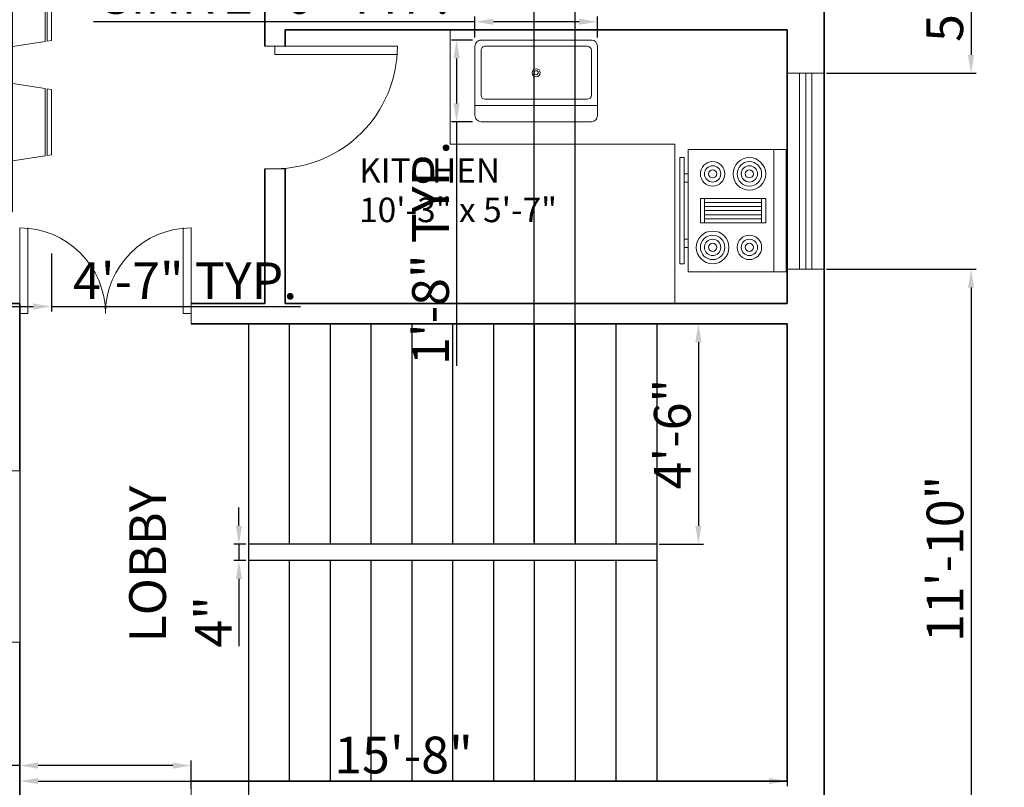
# Model space of a CAD drawing. Units: inches. Extents: x 3087 to 8148, y 1377 to 3709.
# Tile 5 of 6: x 3443 to 3684, y 1689 to 1877. Entities that reach past the tile are written whole.
import ezdxf

# ---------------------------------------------------------------- set-up
doc = ezdxf.new("R2010")
doc.units = ezdxf.units.IN
for name, color, linetype, lineweight, true_color in [('A-ANNO-DIMS', 244, 'Continuous', 18, 0x991b1e), ('A-AREA-IDEN', 244, 'Continuous', 18, 0x991b1e), ('A-DOOR', 146, 'Continuous', 18, 0x105689), ('A-FLOR-STRS', 146, 'Continuous', 25, 0x105689), ('A-GLAZ', 146, 'Continuous', 18, 0x105689), ('A-WALL', 241, 'Continuous', 35, 0xf7abae)]:
    doc.layers.add(name, color=color, linetype=linetype, lineweight=lineweight, true_color=true_color)
for name, color, linetype, lineweight in [('A-EQPM', 8, 'Continuous', 18), ('A-FLOR-CASE', 9, 'Continuous', 18), ('A-FLOR-FIXT', 9, 'Continuous', 18), ('A-FURN', 8, 'Continuous', 18)]:
    doc.layers.add(name, color=color, linetype=linetype, lineweight=lineweight)
doc.styles.get("Standard").update_dxf_attribs({"font": 'arial.ttf'})
doc.dimstyles.new('ISO-25', dxfattribs={"dimtxt": 9, "dimasz": 4.5, "dimexe": 1.25, "dimexo": 0.625, "dimtad": 1, "dimdec": 0, "dimlunit": 3, "dimtxsty": 'Standard', "dimcen": 2.5, "dimadec": 0, "dimazin": 0, "dimtfac": 1, "dimtdec": 0, "dimtmove": 0, "dimatfit": 3, "dimfxl": 1, "dimarcsym": 0})

# ---------------------------------------------------------------- blocks, each defined once
blk = doc.blocks.new('Dining Set - 36 x 72 in.')
for p, q in [((-22, 27.5), (-22.1562, 26.50042)), ((-22, 27.5), (-6, 27.5)), ((-5.8437, 26.49966), (-6, 27.5)), ((6, 27.5), (5.8438, 26.50042)), ((6, 27.5), (22, 27.5)), ((22.1563, 26.49966), (22, 27.5)), ((-22.2343, 26.00059), (-23.4847, 17.99762)), ((-22.2304, 26), (-5.7608, 26)), ((-5.8416, 26.5), (-22.1534, 26.5)), ((-4.5152, 17.99762), (-5.7655, 25.99926)), ((5.7657, 26.00059), (4.5153, 17.99762)), ((5.7696, 26), (22.2392, 26)), ((22.1584, 26.5), (5.8466, 26.5)), ((23.4848, 17.99762), (22.2345, 25.99926)), ((36, 18), (-36, 18)), ((-36, 18), (-36, -18)), ((36, -18), (36, 18)), ((-45.5, 8), (-44.5004, 8.15617)), ((-45.5, 8), (-45.5, -8)), ((-44.5, -8.15843), (-44.5, 8.15338)), ((-44.0006, 8.23428), (-35.9976, 9.48474)), ((-44, 8.23041), (-44, -8.23915)), ((44.0006, 8.23428), (35.9976, 9.48474)), ((44, 8.23041), (44, -8.23915)), ((44.5, -8.15843), (44.5, 8.15338)), ((45.5, 8), (44.5005, 8.15617)), ((45.5, 8), (45.5, -8)), ((-44.4997, -8.15631), (-45.5, -8)), ((-35.9976, -9.48476), (-43.9993, -8.2345)), ((35.9976, -9.48476), (43.9993, -8.2345)), ((44.4997, -8.15631), (45.5, -8)), ((-36, -18), (36, -18)), ((-22.2343, -26.0006), (-23.4847, -17.99762)), ((-4.5152, -17.99762), (-5.7655, -25.99928)), ((5.7657, -26.0006), (4.5153, -17.99762)), ((23.4848, -17.99762), (22.2345, -25.99928)), ((-22.2304, -26), (-5.7608, -26)), ((-22, -27.5), (-22.1562, -26.50044)), ((-5.8416, -26.5), (-22.1534, -26.5)), ((-5.8437, -26.49967), (-6, -27.5)), ((5.7696, -26), (22.2392, -26)), ((6, -27.5), (5.8438, -26.50044)), ((22.1584, -26.5), (5.8466, -26.5)), ((22.1563, -26.49967), (22, -27.5)), ((-22, -27.5), (-6, -27.5)), ((6, -27.5), (22, -27.5))]:
    blk.add_line(p, q)
for points in [[(-36, 15), (-31.1772, 14.97754), (-26.8079, 14.91406), (-22.8538, 14.81543), (-19.276, 14.6875), (-16.0362, 14.53613), (-13.0957, 14.36718), (-10.4159, 14.18652), (-7.9583, 14), (-5.6904, 13.81315), (-3.6035, 13.63021), (-1.6954, 13.45508), (0.0365, 13.29166), (1.5945, 13.14388), (2.9811, 13.01562), (4.1988, 12.9108), (5.25, 12.83333), (6.1393, 12.78613), (6.8802, 12.76823), (7.4883, 12.77767), (7.9792, 12.8125), (8.3685, 12.87077), (8.6719, 12.95052), (8.9049, 13.0498), (9.0833, 13.16666), (9.2205, 13.29899), (9.3216, 13.44401), (9.3895, 13.59879), (9.4271, 13.76041), (9.4373, 13.92594), (9.4232, 14.09245), (9.3875, 14.257), (9.3333, 14.41666), (9.2638, 14.56917), (9.1836, 14.71484), (9.0975, 14.85465), (9.0104, 14.98958), (8.9272, 15.1206), (8.8529, 15.2487), (8.7922, 15.37483), (8.75, 15.5), (8.7305, 15.62467), (8.7344, 15.74739), (8.7617, 15.86621), (8.8125, 15.97916), (8.8867, 16.08431), (8.9844, 16.17968), (9.1055, 16.26334), (9.25, 16.33333), (9.4189, 16.38802), (9.6172, 16.42708), (9.8506, 16.45052), (10.125, 16.45833), (10.4463, 16.45052), (10.8203, 16.42708), (11.2529, 16.38802), (11.75, 16.33333), (12.3184, 16.26318), (12.9694, 16.17838), (13.7151, 16.07991), (14.5677, 15.96875), (15.5395, 15.84586), (16.6426, 15.71224), (17.8893, 15.56884), (19.2917, 15.41666), (20.859, 15.25667), (22.5879, 15.08984), (24.4721, 14.91715), (26.5052, 14.73958), (28.6809, 14.5581), (30.9929, 14.3737), (33.4347, 14.18733), (36, 14)], [(-36, 10), (-28.9766, 10.14274), (-23.1725, 10.20442), (-18.4241, 10.19775), (-14.5677, 10.13541), (-11.4399, 10.03011), (-8.877, 9.89453), (-6.7154, 9.74137), (-4.7917, 9.58333), (-2.9698, 9.43082), (-1.2246, 9.28515), (0.4415, 9.14534), (2.026, 9.01041), (3.5266, 8.87939), (4.9408, 8.7513), (6.266, 8.62516), (7.5, 8.5), (8.6411, 8.37549), (9.6914, 8.2539), (10.6538, 8.13818), (11.5312, 8.03125), (12.3267, 7.93603), (13.043, 7.85547), (13.6831, 7.79248), (14.25, 7.75), (14.7471, 7.7303), (15.1797, 7.73307), (15.5537, 7.75732), (15.875, 7.80208), (16.1494, 7.86637), (16.3828, 7.94922), (16.5811, 8.04964), (16.75, 8.16666), (16.8944, 8.29915), (17.0143, 8.44531), (17.1089, 8.60319), (17.1771, 8.77083), (17.218, 8.94629), (17.2305, 9.1276), (17.2137, 9.31282), (17.1667, 9.5), (17.0895, 9.6875), (16.987, 9.875), (16.8649, 10.0625), (16.7292, 10.25), (16.5856, 10.4375), (16.4401, 10.625), (16.2985, 10.8125), (16.1667, 11), (16.05, 11.18733), (15.9518, 11.3737), (15.8752, 11.5581), (15.8229, 11.73958), (15.798, 11.91715), (15.8034, 12.08984), (15.842, 12.25667), (15.9167, 12.41666), (16.0295, 12.56836), (16.1784, 12.70833), (16.3605, 12.83268), (16.5729, 12.9375), (16.8127, 13.01888), (17.0768, 13.07291), (17.3625, 13.0957), (17.6667, 13.08333), (17.9894, 13.03312), (18.3418, 12.94726), (18.7382, 12.82918), (19.1927, 12.68229), (19.7195, 12.51001), (20.3327, 12.31575), (21.0465, 12.10294), (21.875, 11.875), (22.8357, 11.63354), (23.959, 11.37304), (25.2786, 11.08618), (26.8282, 10.76562), (28.6414, 10.40405), (30.752, 9.99414), (33.1936, 9.52856), (36, 9)], [(-36, 5.5), (-30.7157, 5.3348), (-26.069, 5.20963), (-21.9946, 5.11767), (-18.4271, 5.05208), (-15.3009, 5.00602), (-12.5508, 4.97265), (-10.1112, 4.94515), (-7.9167, 4.91666), (-5.909, 4.88167), (-4.0586, 4.83984), (-2.3429, 4.79215), (-0.7396, 4.73958), (0.7739, 4.6831), (2.22, 4.6237), (3.6213, 4.56233), (5, 4.5), (6.373, 4.43782), (7.7344, 4.3776), (9.0723, 4.32129), (10.375, 4.27083), (11.6309, 4.22819), (12.8281, 4.19531), (13.9551, 4.17415), (15, 4.16666), (15.954, 4.17448), (16.819, 4.19791), (17.6001, 4.23698), (18.3021, 4.29166), (18.9299, 4.36198), (19.4883, 4.44791), (19.9823, 4.54948), (20.4167, 4.66666), (20.7969, 4.79899), (21.1302, 4.94401), (21.4245, 5.09879), (21.6875, 5.26041), (21.9271, 5.42594), (22.1511, 5.59245), (22.3672, 5.757), (22.5834, 5.91666), (22.8065, 6.06868), (23.0404, 6.21093), (23.2879, 6.34147), (23.5521, 6.45833), (23.8358, 6.55957), (24.142, 6.64323), (24.4735, 6.70735), (24.8334, 6.75), (25.2235, 6.76969), (25.642, 6.76692), (26.0858, 6.74267), (26.5521, 6.69791), (27.0379, 6.63362), (27.5404, 6.55078), (28.0565, 6.45036), (28.5834, 6.33333), (29.1242, 6.19987), (29.7071, 6.04687), (30.3661, 5.87044), (31.1354, 5.66666), (32.0493, 5.43164), (33.142, 5.16146), (34.4475, 4.85221), (36, 4.5)], [(-36, -1), (-30.7915, -0.6591), (-26.0195, -0.38216), (-21.6519, -0.16284), (-17.6563, 0.00521), (-14.0005, 0.12833), (-10.6523, 0.21289), (-7.5796, 0.26522), (-4.75, 0.29166), (-2.134, 0.29793), (0.2878, 0.28711), (2.5317, 0.26163), (4.6146, 0.22396), (6.5529, 0.17651), (8.3633, 0.12174), (10.0623, 0.06209), (11.6667, 0), (13.1899, -0.06201), (14.6341, -0.1211), (15.9982, -0.17432), (17.2813, -0.21875), (18.4823, -0.25147), (19.6003, -0.26953), (20.6343, -0.27002), (21.5834, -0.25), (22.4481, -0.20768), (23.2357, -0.14584), (23.9549, -0.06836), (24.6146, 0.02083), (25.2235, 0.11784), (25.7904, 0.21875), (26.3241, 0.31966), (26.8334, 0.41666), (27.3265, 0.50618), (27.8099, 0.58593), (28.2894, 0.65397), (28.7709, 0.70833), (29.2601, 0.74707), (29.763, 0.76823), (30.2855, 0.76985), (30.8334, 0.75), (31.4088, 0.70784), (31.9994, 0.64713), (32.589, 0.57275), (33.1615, 0.48958), (33.7008, 0.4025), (34.1908, 0.3164), (34.6153, 0.23616), (34.9584, 0.16666), (35.2099, 0.11165), (35.3848, 0.07031), (35.504, 0.04069), (35.5886, 0.02083), (35.6594, 0.00879), (35.7377, 0.0026), (35.8442, 0.00032), (36, 0)], [(-36, -6.5), (-27.1843, -6.31267), (-20.084, -6.1263), (-14.469, -5.9419), (-10.1094, -5.76042), (-6.7752, -5.58285), (-4.2363, -5.41016), (-2.2629, -5.24333), (-0.625, -5.08334), (0.8708, -4.93099), (2.2715, -4.78646), (3.5872, -4.64974), (4.8281, -4.52084), (6.0046, -4.39974), (7.127, -4.28646), (8.2053, -4.18099), (9.25, -4.08334), (10.2705, -3.99382), (11.2734, -3.91407), (12.2647, -3.84603), (13.25, -3.79167), (14.2354, -3.75293), (15.2266, -3.73177), (16.2295, -3.73015), (17.25, -3.75), (18.2912, -3.79248), (19.3451, -3.85547), (20.4009, -3.93604), (21.4479, -4.03125), (22.4754, -4.13819), (23.4727, -4.25391), (24.4289, -4.37549), (25.3334, -4.5), (26.1785, -4.62492), (26.9694, -4.74935), (27.7145, -4.87281), (28.4219, -4.99479), (29.1, -5.11483), (29.7572, -5.23242), (30.4016, -5.34709), (31.0417, -5.45834), (31.6837, -5.56437), (32.3262, -5.65821), (32.9658, -5.73153), (33.599, -5.77604), (34.2224, -5.78345), (34.8327, -5.74545), (35.4264, -5.65373), (36, -5.5)], [(-36, -10), (-26.4022, -9.81299), (-18.4675, -9.62891), (-11.9839, -9.45069), (-6.7396, -9.28125), (-2.5226, -9.12354), (0.8789, -8.98047), (3.6769, -8.85498), (6.0833, -8.75), (8.2767, -8.66765), (10.3021, -8.60677), (12.1712, -8.56543), (13.8958, -8.54167), (15.4876, -8.53353), (16.9583, -8.53907), (18.3197, -8.55632), (19.5834, -8.58334), (20.7616, -8.61841), (21.8685, -8.66081), (22.9188, -8.71004), (23.9271, -8.76563), (24.9081, -8.82707), (25.8763, -8.89388), (26.8465, -8.96558), (27.8334, -9.04167), (28.8474, -9.12118), (29.8828, -9.20117), (30.93, -9.27824), (31.9792, -9.34896), (33.0205, -9.40991), (34.0443, -9.45768), (35.0407, -9.48885), (36, -9.5)], [(-36, -14.5), (-30.0881, -14.33513), (-25.0332, -14.21224), (-20.7312, -14.12647), (-17.0781, -14.07292), (-13.97, -14.04671), (-11.3027, -14.04297), (-8.9724, -14.05681), (-6.875, -14.08334), (-4.9224, -14.11833), (-3.0905, -14.16016), (-1.3709, -14.20785), (0.2448, -14.26042), (1.7647, -14.3169), (3.1973, -14.3763), (4.5507, -14.43767), (5.8333, -14.5), (7.0554, -14.5621), (8.235, -14.62175), (9.3922, -14.67652), (10.5469, -14.72396), (11.7192, -14.76164), (12.929, -14.78711), (14.1965, -14.79794), (15.5417, -14.79167), (16.9933, -14.76424), (18.6152, -14.70508), (20.4804, -14.60197), (22.6615, -14.44271), (25.2312, -14.21509), (28.2624, -13.9069), (31.8277, -13.50594), (36, -13)]]:
    blk.add_lwpolyline(points)
blk = doc.blocks.new('Range-Oven - 30 in top')
for p, q in [((0, -3), (30, -3)), ((12, -6), (18, -6)), ((13, -20), (13, -6)), ((14, -6), (14, -20)), ((15, -20), (15, -6)), ((16, -6), (16, -20)), ((17, -20), (17, -6)), ((18, -20), (12, -20)), ((6, -24), (6, -25)), ((8, -25), (8, -24)), ((22, -25), (22, -24)), ((24, -24), (24, -25))]:
    blk.add_line(p, q)
for points in [[(0, -24), (0, 0), (30, 0), (30, -24)], [(12, -21), (12, -5), (18, -5), (18, -21)], [(2, -26), (2, -25), (28, -25), (28, -26)]]:
    blk.add_lwpolyline(points, close=True)
for centre, radius in [((6, -9), 4), ((6, -9), 3), ((6, -9), 2), ((24, -9), 3), ((24, -9), 2), ((6, -9), 1), ((24, -9), 1), ((24, -18), 4), ((6, -18), 3), ((6, -18), 2), ((24, -18), 3), ((24, -18), 2), ((6, -18), 1), ((24, -18), 1)]:
    blk.add_circle(centre, radius)
blk = doc.blocks.new('Sink-single - 30 in top')
blk.add_line((-15, -3.999996), (15, -3.999996))
for points in [[(-13.5, 0), (13.5, 0)], [(-15, -18.499996), (-15, -1.5)], [(15, -1.5), (15, -18.499996)], [(-13.5, -17.499996), (-13.5, -6.499996)], [(-12.5, -5.499996), (12.5, -5.499996)], [(13.5, -6.499996), (13.5, -17.499996)], [(12.5, -18.499996), (-12.5, -18.499996)], [(13.5, -19.999996), (-13.5, -19.999996)]]:
    blk.add_lwpolyline(points)
for radius in [1, 0.5]:
    blk.add_circle((0, -11.999996), radius)
for centre, radius, start, end in [((-13.5, -1.5), 1.5, 90, 180), ((13.5, -1.5), 1.5, 0, 90), ((-12.5, -6.499996), 1, 90, 180), ((12.5, -6.499996), 1, 0, 90), ((-13.5, -18.499996), 1.5, 180, 270), ((-12.5, -17.499996), 1, 180, 270), ((12.5, -17.499996), 1, 270, 0), ((13.5, -18.499996), 1.5, 270, 0)]:
    blk.add_arc(centre, radius, start, end)
blk = doc.blocks.new('*D19')
at = {"layer": 'A-ANNO-DIMS', "color": 0, "lineweight": -2, "transparency": 16777216}
for p, q in [((3442.82, 1703.84), (3442.82, 1689.71)), ((3630.82, 1703.84), (3630.82, 1689.71)), ((3447.32, 1690.96), (3626.32, 1690.96))]:
    blk.add_line(p, q, dxfattribs=at)
at = {"layer": 'A-ANNO-DIMS', "color": 0, "transparency": 16777216}
for points in [[(3447.32, 1691.71), (3447.32, 1690.21), (3442.82, 1690.96)], [(3626.32, 1691.71), (3626.32, 1690.21), (3630.82, 1690.96)]]:
    blk.add_solid(points, dxfattribs=at)
at = {"layer": 'Defpoints', "color": 0, "transparency": 16777216}
for p in [(3442.82, 1704.46), (3630.82, 1704.46), (3630.82, 1690.96)]:
    blk.add_point(p, dxfattribs=at)
at = {"layer": 'A-ANNO-DIMS', "color": 0, "transparency": 16777216, "insert": (3536.82, 1696.18), "char_height": 9, "attachment_point": 5}
blk.add_mtext('15\'-8"', dxfattribs=at)
blk = doc.blocks.new('*D20')
at = {"layer": 'A-ANNO-DIMS', "color": 0, "lineweight": -2, "transparency": 16777216}
for p, q in [((3599.44, 1802.96), (3610.28, 1802.96)), ((3609.03, 1798.46), (3609.03, 1753.46)), ((3599.44, 1748.96), (3610.28, 1748.96))]:
    blk.add_line(p, q, dxfattribs=at)
at = {"layer": 'A-ANNO-DIMS', "color": 0, "transparency": 16777216}
for points in [[(3608.28, 1798.46), (3609.78, 1798.46), (3609.03, 1802.96)], [(3608.28, 1753.46), (3609.78, 1753.46), (3609.03, 1748.96)]]:
    blk.add_solid(points, dxfattribs=at)
at = {"layer": 'Defpoints', "color": 0, "transparency": 16777216}
for p in [(3598.82, 1802.96), (3598.82, 1748.96), (3609.03, 1748.96)]:
    blk.add_point(p, dxfattribs=at)
at = {"layer": 'A-ANNO-DIMS', "color": 0, "transparency": 16777216, "insert": (3603.81, 1775.96), "char_height": 9, "attachment_point": 5, "rotation": 90}
blk.add_mtext('4\'-6"', dxfattribs=at)
blk = doc.blocks.new('*D21')
at = {"layer": 'A-ANNO-DIMS', "color": 0, "lineweight": -2, "transparency": 16777216}
for p, q in [((3496.51, 1753.46), (3496.51, 1757.96)), ((3498.19, 1748.96), (3495.26, 1748.96)), ((3496.51, 1748.96), (3496.51, 1744.96)), ((3498.19, 1744.96), (3495.26, 1744.96)), ((3496.51, 1740.46), (3496.51, 1724))]:
    blk.add_line(p, q, dxfattribs=at)
at = {"layer": 'A-ANNO-DIMS', "color": 0, "transparency": 16777216}
for points in [[(3495.76, 1753.46), (3497.26, 1753.46), (3496.51, 1748.96)], [(3495.76, 1740.46), (3497.26, 1740.46), (3496.51, 1744.96)]]:
    blk.add_solid(points, dxfattribs=at)
at = {"layer": 'Defpoints', "color": 0, "transparency": 16777216}
for p in [(3498.82, 1748.96), (3496.51, 1744.96), (3498.82, 1744.96)]:
    blk.add_point(p, dxfattribs=at)
at = {"layer": 'A-ANNO-DIMS', "color": 0, "transparency": 16777216, "insert": (3491.38, 1729.98), "char_height": 9, "attachment_point": 5, "rotation": 90}
blk.add_mtext('4"', dxfattribs=at)
blk = doc.blocks.new('DOOR-SINGLE-30IN')
for p, q in [((0, 30), (30, 30)), ((30, 30), (30, 28)), ((0, 28), (30, 28))]:
    blk.add_line(p, q)
blk.add_arc((30, 30), 30, 180, 270)
blk = doc.blocks.new('DOOR-DOUBLE-42IN')
for p, q in [((0, 21), (0, 0)), ((2, 21), (2, 0)), ((40, 21), (40, 0)), ((42, 21), (42, 0)), ((0, 0), (2, 0)), ((42, 0), (40, 0))]:
    blk.add_line(p, q)
for centre, start, end in [((0, 0), 0, 90), ((42, 0), 90, 180)]:
    blk.add_arc(centre, 21, start, end)
blk = doc.blocks.new('WINDOW-48IN')
for p, q in [((0, 0), (0, 48)), ((0, 48), (9, 48)), ((3, 0), (3, 48)), ((4.5, 0), (4.5, 48)), ((6, 0), (6, 48)), ((9, 48), (9, 0)), ((9, 0), (0, 0))]:
    blk.add_line(p, q)
blk = doc.blocks.new('*D42')
at = {"layer": 'A-ANNO-DIMS', "color": 0, "lineweight": -2, "transparency": 16777216}
for p, q in [((3395.58, 1820.23), (3395.58, 1805.96)), ((3450.58, 1820.23), (3450.58, 1805.96)), ((3400.08, 1807.21), (3446.08, 1807.21)), ((3450.58, 1807.21), (3511.55, 1807.21))]:
    blk.add_line(p, q, dxfattribs=at)
at = {"layer": 'A-ANNO-DIMS', "color": 0, "transparency": 16777216}
for points in [[(3400.08, 1807.96), (3400.08, 1806.46), (3395.58, 1807.21)], [(3446.08, 1807.96), (3446.08, 1806.46), (3450.58, 1807.21)]]:
    blk.add_solid(points, dxfattribs=at)
at = {"layer": 'Defpoints', "color": 0, "transparency": 16777216}
for p in [(3395.58, 1820.86), (3450.58, 1820.86), (3450.58, 1807.21)]:
    blk.add_point(p, dxfattribs=at)
at = {"layer": 'A-ANNO-DIMS', "color": 0, "transparency": 16777216, "insert": (3483.32, 1812.34), "char_height": 9, "attachment_point": 5}
blk.add_mtext('4\'-7" TYP.', dxfattribs=at)
blk = doc.blocks.new('*D47')
at = {"layer": 'A-ANNO-DIMS', "color": 0, "lineweight": -2, "transparency": 16777216}
for p, q in [((3554.32, 1876.96), (3460.91, 1876.96)), ((3554.32, 1873.09), (3554.32, 1878.21)), ((3579.82, 1876.96), (3558.82, 1876.96)), ((3584.32, 1873.09), (3584.32, 1878.21))]:
    blk.add_line(p, q, dxfattribs=at)
at = {"layer": 'A-ANNO-DIMS', "color": 0, "transparency": 16777216}
for points in [[(3558.82, 1877.71), (3558.82, 1876.21), (3554.32, 1876.96)], [(3579.82, 1877.71), (3579.82, 1876.21), (3584.32, 1876.96)]]:
    blk.add_solid(points, dxfattribs=at)
at = {"layer": 'Defpoints', "color": 0, "transparency": 16777216}
for p in [(3554.32, 1876.96), (3554.32, 1872.46), (3584.32, 1872.46)]:
    blk.add_point(p, dxfattribs=at)
at = {"layer": 'A-ANNO-DIMS', "color": 0, "transparency": 16777216, "insert": (3505.37, 1882.24), "char_height": 9, "attachment_point": 5}
blk.add_mtext('SINK 2\'-6" TYP.', dxfattribs=at)
blk = doc.blocks.new('*D48')
at = {"layer": 'A-ANNO-DIMS', "color": 0, "lineweight": -2, "transparency": 16777216}
for p, q in [((3553.69, 1872.46), (3548.57, 1872.46)), ((3549.82, 1867.96), (3549.82, 1856.96)), ((3553.69, 1852.46), (3548.57, 1852.46)), ((3549.82, 1852.46), (3549.82, 1792.7))]:
    blk.add_line(p, q, dxfattribs=at)
at = {"layer": 'A-ANNO-DIMS', "color": 0, "transparency": 16777216}
for points in [[(3549.07, 1867.96), (3550.57, 1867.96), (3549.82, 1872.46)], [(3549.07, 1856.96), (3550.57, 1856.96), (3549.82, 1852.46)]]:
    blk.add_solid(points, dxfattribs=at)
at = {"layer": 'Defpoints', "color": 0, "transparency": 16777216}
for p in [(3554.32, 1872.46), (3549.82, 1852.46), (3554.32, 1852.46)]:
    blk.add_point(p, dxfattribs=at)
at = {"layer": 'A-ANNO-DIMS', "color": 0, "transparency": 16777216, "insert": (3544.6, 1820.33), "char_height": 9, "attachment_point": 5, "rotation": 90}
blk.add_mtext('1\'-8" TYP.', dxfattribs=at)
blk = doc.blocks.new('*D49')
at = {"layer": 'A-ANNO-DIMS', "color": 0, "lineweight": -2, "transparency": 16777216}
for p, q in [((3442.82, 1689.09), (3442.82, 1696.01)), ((3484.82, 1689.09), (3484.82, 1696.01)), ((3442.82, 1694.76), (3286.25, 1694.76)), ((3480.32, 1694.76), (3447.32, 1694.76))]:
    blk.add_line(p, q, dxfattribs=at)
at = {"layer": 'A-ANNO-DIMS', "color": 0, "transparency": 16777216}
for points in [[(3447.32, 1695.51), (3447.32, 1694.01), (3442.82, 1694.76)], [(3480.32, 1695.51), (3480.32, 1694.01), (3484.82, 1694.76)]]:
    blk.add_solid(points, dxfattribs=at)
at = {"layer": 'Defpoints', "color": 0, "transparency": 16777216}
for p in [(3442.82, 1694.76), (3442.82, 1688.46), (3484.82, 1688.46)]:
    blk.add_point(p, dxfattribs=at)
at = {"layer": 'A-ANNO-DIMS', "color": 0, "transparency": 16777216, "insert": (3362.28, 1700.05), "char_height": 9, "attachment_point": 5}
blk.add_mtext('DOUBLE DOOR 3\'-6" TYP.', dxfattribs=at)
blk = doc.blocks.new('*D66')
at = {"layer": 'A-ANNO-DIMS', "color": 0, "lineweight": -2, "transparency": 16777216}
for p, q in [((3640.44, 1934.82), (3677.07, 1934.82)), ((3675.82, 1930.32), (3675.82, 1868.83)), ((3640.44, 1864.33), (3677.07, 1864.33))]:
    blk.add_line(p, q, dxfattribs=at)
at = {"layer": 'A-ANNO-DIMS', "color": 0, "transparency": 16777216}
for points in [[(3675.07, 1930.32), (3676.57, 1930.32), (3675.82, 1934.82)], [(3675.07, 1868.83), (3676.57, 1868.83), (3675.82, 1864.33)]]:
    blk.add_solid(points, dxfattribs=at)
at = {"layer": 'Defpoints', "color": 0, "transparency": 16777216}
for p in [(3639.82, 1934.82), (3639.82, 1864.33), (3675.82, 1864.33)]:
    blk.add_point(p, dxfattribs=at)
at = {"layer": 'A-ANNO-DIMS', "color": 0, "transparency": 16777216, "insert": (3670.54, 1899.58), "char_height": 9, "attachment_point": 5, "rotation": 90}
blk.add_mtext('5\'-10 1/2"', dxfattribs=at)
blk = doc.blocks.new('*D67')
at = {"layer": 'A-ANNO-DIMS', "color": 0, "lineweight": -2, "transparency": 16777216}
for p, q in [((3640.44, 1816.33), (3677.07, 1816.33)), ((3675.82, 1811.83), (3675.82, 1678.99)), ((3640.44, 1674.49), (3677.07, 1674.49))]:
    blk.add_line(p, q, dxfattribs=at)
at = {"layer": 'A-ANNO-DIMS', "color": 0, "transparency": 16777216}
for points in [[(3675.07, 1811.83), (3676.57, 1811.83), (3675.82, 1816.33)], [(3675.07, 1678.99), (3676.57, 1678.99), (3675.82, 1674.49)]]:
    blk.add_solid(points, dxfattribs=at)
at = {"layer": 'Defpoints', "color": 0, "transparency": 16777216}
for p in [(3639.82, 1816.33), (3639.82, 1674.49), (3675.82, 1674.49)]:
    blk.add_point(p, dxfattribs=at)
at = {"layer": 'A-ANNO-DIMS', "color": 0, "transparency": 16777216, "insert": (3670.6, 1745.41), "char_height": 9, "attachment_point": 5, "rotation": 90}
blk.add_mtext('11\'-10"', dxfattribs=at)
blk = doc.blocks.new('*D69')
at = {"layer": 'A-ANNO-DIMS', "color": 0, "lineweight": -2, "transparency": 16777216}
for p, q in [((3442.82, 1804.84), (3442.82, 1376.71)), ((3498.82, 1802.34), (3498.82, 1376.71)), ((3447.32, 1377.96), (3494.32, 1377.96))]:
    blk.add_line(p, q, dxfattribs=at)
at = {"layer": 'A-ANNO-DIMS', "color": 0, "transparency": 16777216}
for points in [[(3447.32, 1378.71), (3447.32, 1377.21), (3442.82, 1377.96)], [(3494.32, 1378.71), (3494.32, 1377.21), (3498.82, 1377.96)]]:
    blk.add_solid(points, dxfattribs=at)
at = {"layer": 'Defpoints', "color": 0, "transparency": 16777216}
for p in [(3442.82, 1805.46), (3498.82, 1802.96), (3498.82, 1377.96)]:
    blk.add_point(p, dxfattribs=at)
at = {"layer": 'A-ANNO-DIMS', "color": 0, "transparency": 16777216, "insert": (3470.82, 1383.18), "char_height": 9, "attachment_point": 5}
blk.add_mtext('4\'-8"', dxfattribs=at)
blk = doc.blocks.new('*D70')
at = {"layer": 'A-ANNO-DIMS', "color": 0, "lineweight": -2, "transparency": 16777216}
for p, q in [((3568.82, 1749.59), (3568.82, 2111.21)), ((3578.82, 1749.59), (3578.82, 2111.21)), ((3564.32, 2109.96), (3559.82, 2109.96)), ((3568.82, 2109.96), (3578.82, 2109.96)), ((3583.32, 2109.96), (3619.98, 2109.96))]:
    blk.add_line(p, q, dxfattribs=at)
at = {"layer": 'A-ANNO-DIMS', "color": 0, "transparency": 16777216}
for points in [[(3564.32, 2110.71), (3564.32, 2109.21), (3568.82, 2109.96)], [(3583.32, 2110.71), (3583.32, 2109.21), (3578.82, 2109.96)]]:
    blk.add_solid(points, dxfattribs=at)
at = {"layer": 'Defpoints', "color": 0, "transparency": 16777216}
for p in [(3578.82, 2109.96), (3568.82, 1748.96), (3578.82, 1748.96)]:
    blk.add_point(p, dxfattribs=at)
at = {"layer": 'A-ANNO-DIMS', "color": 0, "transparency": 16777216, "insert": (3603.9, 2115.18), "char_height": 9, "attachment_point": 5}
blk.add_mtext('0\'-10"', dxfattribs=at)

msp = doc.modelspace()

# ---------------------------------------------------------------- linework, layer by layer
at = {"layer": 'A-DOOR'}
for p, q in [((3502.82, 1870.96), (3507.82, 1870.96)), ((3502.82, 1840.96), (3507.82, 1840.96)), ((3484.82, 1802.96), (3484.82, 1807.96)), ((3442.82, 1766.96), (3437.82, 1766.96)), ((3442.82, 1724.96), (3437.82, 1724.96)), ((3484.82, 1685.96), (3484.82, 1690.96))]:
    msp.add_line(p, q, dxfattribs=at)
at = {"layer": 'A-FLOR-CASE'}
for p, q in [((3548.26, 1846.96), (3548.26, 1874.96)), ((3548.26, 1846.96), (3603.28, 1846.96)), ((3603.28, 1846.96), (3603.28, 1807.96))]:
    msp.add_line(p, q, dxfattribs=at)
at = {"layer": 'A-FLOR-STRS'}
for p, q in [((3498.82, 1802.96), (3498.82, 1690.96)), ((3508.82, 1802.96), (3508.82, 1748.96)), ((3518.82, 1802.96), (3518.82, 1748.96)), ((3528.82, 1802.96), (3528.82, 1748.96)), ((3538.82, 1802.96), (3538.82, 1748.96)), ((3548.82, 1802.96), (3548.82, 1748.96)), ((3558.82, 1802.96), (3558.82, 1748.96)), ((3568.82, 1802.96), (3568.82, 1748.96)), ((3578.82, 1802.96), (3578.82, 1748.96)), ((3588.82, 1802.96), (3588.82, 1748.96)), ((3598.82, 1802.96), (3598.82, 1690.96)), ((3598.82, 1748.96), (3498.82, 1748.96)), ((3598.82, 1744.96), (3498.82, 1744.96)), ((3508.82, 1744.96), (3508.82, 1690.96)), ((3518.82, 1744.96), (3518.82, 1690.96)), ((3528.82, 1744.96), (3528.82, 1690.96)), ((3538.82, 1744.96), (3538.82, 1690.96)), ((3548.82, 1744.96), (3548.82, 1690.96)), ((3558.82, 1744.96), (3558.82, 1690.96)), ((3568.82, 1744.96), (3568.82, 1690.96)), ((3578.82, 1744.96), (3578.82, 1690.96)), ((3588.82, 1744.96), (3588.82, 1690.96))]:
    msp.add_line(p, q, dxfattribs=at)
at = {"layer": 'A-WALL'}
for p, q in [((3639.82, 2073.96), (3639.82, 1413.96)), ((3502.82, 1870.96), (3502.82, 1885.96)), ((3507.82, 1874.96), (3630.82, 1874.96)), ((3507.82, 1870.96), (3507.82, 1874.96)), ((3630.82, 1874.96), (3630.82, 1807.96)), ((3502.82, 1807.96), (3502.82, 1840.96)), ((3507.82, 1807.96), (3507.82, 1840.96)), ((3382.82, 1807.96), (3442.82, 1807.96)), ((3442.82, 1766.96), (3442.82, 1807.96)), ((3484.82, 1807.96), (3496.82, 1807.96)), ((3496.82, 1807.96), (3502.82, 1807.96)), ((3507.82, 1807.96), (3630.82, 1807.96)), ((3484.82, 1802.96), (3496.82, 1802.96)), ((3496.82, 1802.96), (3630.82, 1802.96)), ((3502.82, 1802.96), (3507.82, 1802.96)), ((3630.82, 1802.96), (3630.82, 1690.96)), ((3442.82, 1683.96), (3442.82, 1724.96)), ((3630.82, 1690.96), (3484.82, 1690.96))]:
    msp.add_line(p, q, dxfattribs=at)

# ---------------------------------------------------------------- block references
at = {"layer": 'A-DOOR', "extrusion": (0, 0, -1), "zscale": -1}
msp.add_blockref('DOOR-SINGLE-30IN', (-3535.32, 1840.96), dxfattribs=at)
at = {"layer": 'A-DOOR'}
msp.add_blockref('DOOR-DOUBLE-42IN', (3442.82, 1805.46), dxfattribs=at)
at = {"layer": 'A-EQPM', "rotation": 270}
msp.add_blockref('Range-Oven - 30 in top', (3630.53, 1845.69), dxfattribs=at)
at = {"layer": 'A-FLOR-FIXT', "rotation": 180}
msp.add_blockref('Sink-single - 30 in top', (3569.32, 1852.46), dxfattribs=at)
at = {"layer": 'A-FURN', "rotation": 269.9999999999999}
msp.add_blockref('Dining Set - 36 x 72 in.', (3423.08, 1866.36), dxfattribs=at)
at = {"layer": 'A-GLAZ'}
msp.add_blockref('WINDOW-48IN', (3630.82, 1816.33), dxfattribs=at)

# ---------------------------------------------------------------- texts
at = {"layer": 'A-AREA-IDEN'}
for s, p in [('KITCHEN', (3525.95, 1837.51)), ('10\'-3" x 5\'-7"', (3525.95, 1827.87))]:
    msp.add_text(s, height=6, dxfattribs=at).set_placement(p)
msp.add_text('LOBBY ', height=9, rotation=90, dxfattribs=at).set_placement((3478.64, 1724.9))

# ---------------------------------------------------------------- dimensions: what is measured, and where the dimension line sits
at = {"layer": 'A-ANNO-DIMS'}
for base, p1, p2, override, picture, middle in [((3578.82, 2109.96), (3568.82, 1748.96), (3578.82, 1748.96), {"dimdec": 1, "dimlfac": 1, "dimrnd": 0, "dimzin": 1, "dimdsep": 46, "dimlunit": 4, "dimfrac": 2}, '*D70', (3603.9, 2115.18)), ((3498.82, 1377.96), (3442.82, 1805.46), (3498.82, 1802.96), {"dimdec": 1, "dimlfac": 1, "dimrnd": 0, "dimzin": 1, "dimdsep": 46, "dimlunit": 4, "dimfrac": 2}, '*D69', (3470.82, 1383.18)), ((3630.82, 1690.96), (3442.82, 1704.46), (3630.82, 1704.46), {"dimclrd": 0, "dimclre": 0, "dimclrt": 0}, '*D19', (3536.82, 1696.18))]:
    dim = msp.add_linear_dim(base=base, p1=p1, p2=p2, dimstyle='ISO-25', override=override, dxfattribs=at)
    dim.commit()
    dim.dimension.update_dxf_attribs({"geometry": picture, "text_midpoint": middle})
for base, p1, p2, override, picture, middle in [((3675.82, 1864.33), (3639.82, 1934.82), (3639.82, 1864.33), {"dimdec": 1, "dimlfac": 1, "dimrnd": 0, "dimzin": 1, "dimdsep": 46, "dimlunit": 4, "dimfrac": 2}, '*D66', (3670.54, 1899.58)), ((3675.82, 1674.49), (3639.82, 1816.33), (3639.82, 1674.49), {"dimdec": 1, "dimlfac": 1, "dimrnd": 0, "dimzin": 1, "dimdsep": 46, "dimlunit": 4, "dimfrac": 2}, '*D67', (3670.6, 1745.41)), ((3609.03, 1748.96), (3598.82, 1802.96), (3598.82, 1748.96), {"dimclrd": 0, "dimclre": 0, "dimclrt": 0}, '*D20', (3603.81, 1775.96)), ((3496.51, 1744.96), (3498.82, 1748.96), (3498.82, 1744.96), {"dimclrd": 0, "dimclre": 0, "dimclrt": 0}, '*D21', (3491.38, 1729.98))]:
    dim = msp.add_linear_dim(base=base, p1=p1, p2=p2, angle=90, dimstyle='ISO-25', override=override, dxfattribs=at)
    dim.commit()
    dim.dimension.update_dxf_attribs({"geometry": picture, "text_midpoint": middle})
for base, p1, p2, angle, text, picture, middle in [((3554.32, 1876.96), (3584.32, 1872.46), (3554.32, 1872.46), 180, 'SINK <> TYP.', '*D47', (3505.37, 1882.24)), ((3549.82, 1852.46), (3554.32, 1872.46), (3554.32, 1852.46), 270, '<> TYP.', '*D48', (3544.6, 1820.33)), ((3442.82, 1694.76), (3484.82, 1688.46), (3442.82, 1688.46), 180, 'DOUBLE DOOR <> TYP.', '*D49', (3362.28, 1700.05))]:
    dim = msp.add_linear_dim(base=base, p1=p1, p2=p2, angle=angle, text=text, dimstyle='ISO-25', override={"dimdec": 1, "dimlfac": 1, "dimrnd": 0, "dimzin": 1, "dimdsep": 46, "dimlunit": 4, "dimfrac": 2}, dxfattribs=at)
    dim.commit()
    dim.dimension.update_dxf_attribs({"geometry": picture, "text_midpoint": middle})
dim = msp.add_linear_dim(base=(3450.58, 1807.21), p1=(3395.58, 1820.86), p2=(3450.58, 1820.86), text='<> TYP.', dimstyle='ISO-25', override={"dimdec": 1, "dimlfac": 1, "dimrnd": 0, "dimzin": 1, "dimdsep": 46, "dimlunit": 4, "dimfrac": 2}, dxfattribs=at)
dim.commit()
dim.dimension.update_dxf_attribs({"geometry": '*D42', "text_midpoint": (3483.32, 1812.34)})

doc.saveas('drawing.dxf')
